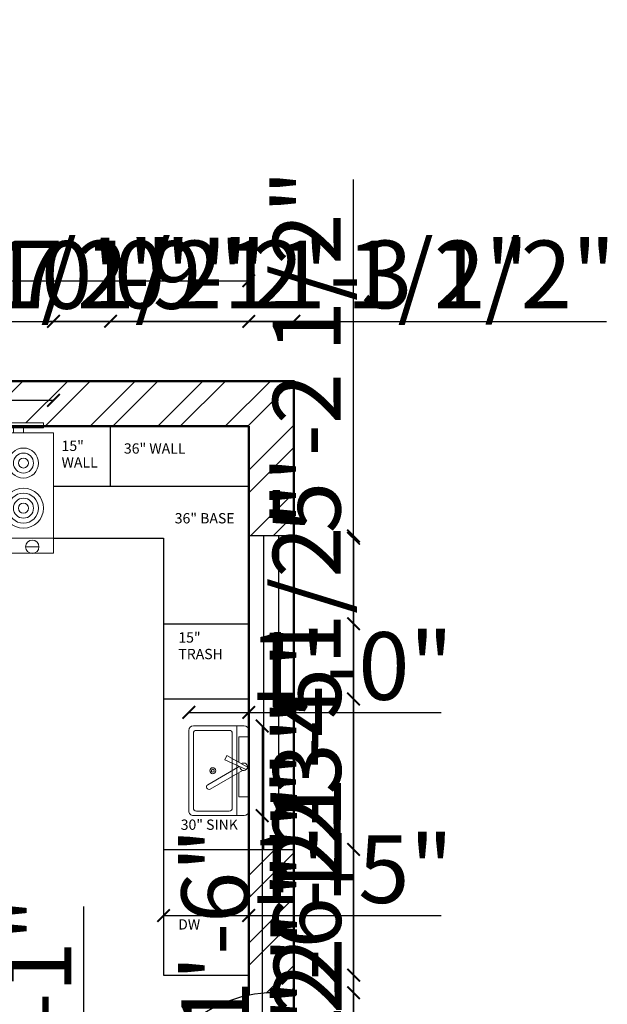
# Model space of a CAD drawing. Units: inches. Extents: x 1736 to 2023, y 1717 to 2014.
# Tile 3 of 3: x 1906 to 2023, y 1818 to 2014. Entities that reach past the tile are written whole.
import ezdxf

# ---------------------------------------------------------------- set-up
doc = ezdxf.new("R2010")
doc.units = ezdxf.units.IN
for name, color, linetype, lineweight in [('A-ANNO-DIMS', 2, 'Continuous', 18), ('A-ANNO-TEXT', 3, 'Continuous', 18), ('A-DOOR', 4, 'Continuous', 25), ('A-EQPM', 9, 'Continuous', 18), ('A-FLOR-CASE', 8, 'Continuous', 25), ('A-FLOR-FIXT', 9, 'Continuous', 18), ('A-GLAZ', 4, 'Continuous', 25), ('A-WALL', 7, 'Continuous', 50), ('A-WALL-PATT', 8, 'Continuous', 13)]:
    doc.layers.add(name, color=color, linetype=linetype, lineweight=lineweight)
doc.styles.get("Standard").update_dxf_attribs({"font": 'arial.ttf'})
doc.dimstyles.new('ISO-25', dxfattribs={"dimtxt": 13.5, "dimasz": 2.5, "dimexe": 1.25, "dimexo": 0.625, "dimtad": 1, "dimdec": 0, "dimlunit": 4, "dimtxsty": 'Standard', "dimblk": 'ARCHTICK', "dimcen": 2.5, "dimse1": 1, "dimse2": 1, "dimclrd": 2, "dimclrt": 4, "dimadec": 0, "dimazin": 0, "dimtfac": 1, "dimtdec": 0, "dimtmove": 0, "dimatfit": 3, "dimfxl": 1, "dimarcsym": 0})

# ---------------------------------------------------------------- blocks, each defined once
blk = doc.blocks.new('Range-Oven - 30 in top')
for p, q in [((0, -3), (30, -3)), ((12, -6), (18, -6)), ((13, -20), (13, -6)), ((14, -6), (14, -20)), ((15, -20), (15, -6)), ((16, -6), (16, -20)), ((17, -20), (17, -6)), ((18, -20), (12, -20)), ((6, -24), (6, -25)), ((8, -25), (8, -24)), ((22, -25), (22, -24)), ((24, -24), (24, -25))]:
    blk.add_line(p, q)
for points in [[(0, -24), (0, 0), (30, 0), (30, -24)], [(12, -21), (12, -5), (18, -5), (18, -21)], [(2, -26), (2, -25), (28, -25), (28, -26)]]:
    blk.add_lwpolyline(points, close=True)
for centre, radius in [((6, -9), 4), ((6, -9), 3), ((6, -9), 2), ((24, -9), 3), ((24, -9), 2), ((6, -9), 1), ((24, -9), 1), ((6, -18), 3), ((24, -18), 4), ((24, -18), 3), ((6, -18), 2), ((6, -18), 1), ((24, -18), 2), ((24, -18), 1)]:
    blk.add_circle(centre, radius)
blk = doc.blocks.new('*U4')
for p, q in [((0, 0), (0, -6)), ((40, 0), (40, -6))]:
    blk.add_line(p, q)
blk.add_lwpolyline([(0, 0), (0, 40), (1.75, 40), (1.75, 0)], close=True)
blk.add_arc((0, 0), 40, 0, 90)
blk = doc.blocks.new('Sink-single - 30 in top')
blk.add_line((-15, -3.999996), (15, -3.999996))
for points in [[(-13.5, 0), (13.5, 0)], [(-15, -18.499996), (-15, -1.5)], [(15, -1.5), (15, -18.499996)], [(-13.5, -17.499996), (-13.5, -6.499996)], [(-12.5, -5.499996), (12.5, -5.499996)], [(13.5, -6.499996), (13.5, -17.499996)], [(12.5, -18.499996), (-12.5, -18.499996)], [(13.5, -19.999996), (-13.5, -19.999996)]]:
    blk.add_lwpolyline(points)
for radius in [1, 0.5]:
    blk.add_circle((0, -11.999996), radius)
for centre, radius, start, end in [((-13.5, -1.5), 1.5, 90, 180), ((13.5, -1.5), 1.5, 0, 90), ((-12.5, -6.499996), 1, 90, 180), ((12.5, -6.499996), 1, 0, 90), ((-13.5, -18.499996), 1.5, 180, 270), ((-12.5, -17.499996), 1, 180, 270), ((12.5, -17.499996), 1, 270, 0), ((13.5, -18.499996), 1.5, 270, 0)]:
    blk.add_arc(centre, radius, start, end)
blk = doc.blocks.new('Faucet - single handle top')
for p, q in [((0.08, -0.26), (-2.26, -4.34)), ((-1.37, -4.79), (0.55, -0.5)), ((-0.06, -1.9), (3.57, -8.18)), ((4.43, -7.68), (0.72, -1.24)), ((-2.26, -4.34), (-1.37, -4.79))]:
    blk.add_line(p, q)
for points in [[(-0.92, -2), (-6, -2), (-6, 0), (6, 0), (6, -2), (1.16, -2)], [(-0.01, -2), (-0.12, -2)]]:
    blk.add_lwpolyline(points)
for centre, radius, start, end in [((0, -1), 0.75, 269.2246, 216.2304), ((4, -7.93), 0.5, 210, 30)]:
    blk.add_arc(centre, radius, start, end)
blk = doc.blocks.new('_ArchTick')
at = {"color": 0, "linetype": 'ByBlock', "const_width": 0.15}
blk.add_lwpolyline([(-0.5, -0.5), (0.5, 0.5)], dxfattribs=at)
blk = doc.blocks.new('*D7')
at = {"layer": 'A-ANNO-DIMS', "color": 0, "lineweight": -2, "transparency": 16777216}
blk.add_line((1831.43, 1962.29), (1951.43, 1962.29), dxfattribs=at)
at = {"layer": 'Defpoints', "color": 0, "transparency": 16777216}
for p in [(1951.43, 1962.29), (1831.43, 1933.29), (1951.43, 1933.29)]:
    blk.add_point(p, dxfattribs=at)
at = {"layer": 'A-ANNO-DIMS', "color": 0, "lineweight": -2, "transparency": 16777216, "xscale": 2.5, "yscale": 2.5, "zscale": 2.5, "rotation": 180}
blk.add_blockref('_ArchTick', (1831.43, 1962.29), dxfattribs=at)
at = {"layer": 'A-ANNO-DIMS', "color": 0, "lineweight": -2, "transparency": 16777216, "xscale": 2.5, "yscale": 2.5, "zscale": 2.5}
blk.add_blockref('_ArchTick', (1951.43, 1962.29), dxfattribs=at)
at = {"layer": 'A-ANNO-DIMS', "color": 0, "transparency": 16777216, "insert": (1891.43, 1969.8), "char_height": 13.5, "attachment_point": 5}
blk.add_mtext("10'", dxfattribs=at)
blk = doc.blocks.new('*D9')
at = {"layer": 'A-ANNO-DIMS', "color": 2, "lineweight": -2, "transparency": 16777216}
for p, q in [((1882.52, 1938.43), (1771.27, 1938.43)), ((1912.52, 1938.43), (1882.52, 1938.43))]:
    blk.add_line(p, q, dxfattribs=at)
at = {"layer": 'Defpoints', "color": 0, "transparency": 16777216}
for p in [(1882.52, 1938.43), (1882.52, 1933.93), (1912.52, 1933.93)]:
    blk.add_point(p, dxfattribs=at)
at = {"layer": 'A-ANNO-DIMS', "color": 2, "lineweight": -2, "transparency": 16777216, "xscale": 2.5, "yscale": 2.5, "zscale": 2.5, "rotation": 180}
blk.add_blockref('_ArchTick', (1882.52, 1938.43), dxfattribs=at)
at = {"layer": 'A-ANNO-DIMS', "color": 2, "lineweight": -2, "transparency": 16777216, "xscale": 2.5, "yscale": 2.5, "zscale": 2.5}
blk.add_blockref('_ArchTick', (1912.52, 1938.43), dxfattribs=at)
at = {"layer": 'A-ANNO-DIMS', "color": 4, "transparency": 16777216, "insert": (1825.64, 1946.04), "char_height": 13.5, "attachment_point": 5}
blk.add_mtext('RANGE 2\'-6"', dxfattribs=at)
blk = doc.blocks.new('*D11')
at = {"layer": 'A-ANNO-DIMS', "color": 2, "lineweight": -2, "transparency": 16777216}
for p, q in [((1954.12, 1873.5), (1954.12, 1855.61)), ((1954.12, 1855.61), (1954.12, 1766.78))]:
    blk.add_line(p, q, dxfattribs=at)
at = {"layer": 'Defpoints', "color": 0, "transparency": 16777216}
for p in [(1951.43, 1873.5), (1951.43, 1855.61), (1954.12, 1855.61)]:
    blk.add_point(p, dxfattribs=at)
at = {"layer": 'A-ANNO-DIMS', "color": 2, "lineweight": -2, "transparency": 16777216, "xscale": 2.5, "yscale": 2.5, "zscale": 2.5}
for p, rotation in [((1954.12, 1873.5), 90), ((1954.12, 1855.61), 270)]:
    blk.add_blockref('_ArchTick', p, dxfattribs=dict(at, rotation=rotation))
at = {"layer": 'A-ANNO-DIMS', "color": 4, "transparency": 16777216, "insert": (1946.51, 1809.94), "char_height": 13.5, "attachment_point": 5, "rotation": 90}
blk.add_mtext('SINK 1\'-6"', dxfattribs=at)
blk = doc.blocks.new('*D12')
at = {"layer": 'A-ANNO-DIMS', "color": 2, "lineweight": -2, "transparency": 16777216}
for p, q in [((1939.5, 1876.19), (1951.43, 1876.19)), ((1951.43, 1876.19), (1989.8, 1876.19))]:
    blk.add_line(p, q, dxfattribs=at)
at = {"layer": 'Defpoints', "color": 0, "transparency": 16777216}
for p in [(1951.43, 1876.19), (1939.5, 1873.5), (1951.43, 1873.5)]:
    blk.add_point(p, dxfattribs=at)
at = {"layer": 'A-ANNO-DIMS', "color": 2, "lineweight": -2, "transparency": 16777216, "xscale": 2.5, "yscale": 2.5, "zscale": 2.5, "rotation": 180}
blk.add_blockref('_ArchTick', (1939.5, 1876.19), dxfattribs=at)
at = {"layer": 'A-ANNO-DIMS', "color": 2, "lineweight": -2, "transparency": 16777216, "xscale": 2.5, "yscale": 2.5, "zscale": 2.5}
blk.add_blockref('_ArchTick', (1951.43, 1876.19), dxfattribs=at)
at = {"layer": 'A-ANNO-DIMS', "color": 4, "transparency": 16777216, "insert": (1971.87, 1883.7), "char_height": 13.5, "attachment_point": 5}
blk.add_mtext('1\'-0"', dxfattribs=at)
blk = doc.blocks.new('*D16')
at = {"layer": 'A-ANNO-DIMS', "color": 2, "lineweight": -2, "transparency": 16777216}
for p, q in [((1951.43, 1954.19), (1911.8, 1954.19)), ((1960.43, 1954.19), (1951.43, 1954.19))]:
    blk.add_line(p, q, dxfattribs=at)
at = {"layer": 'Defpoints', "color": 0, "transparency": 16777216}
for p in [(1951.43, 1954.19), (1960.43, 1942.29), (1951.43, 1933.29)]:
    blk.add_point(p, dxfattribs=at)
at = {"layer": 'A-ANNO-DIMS', "color": 2, "lineweight": -2, "transparency": 16777216, "xscale": 2.5, "yscale": 2.5, "zscale": 2.5, "rotation": 180}
blk.add_blockref('_ArchTick', (1951.43, 1954.19), dxfattribs=at)
at = {"layer": 'A-ANNO-DIMS', "color": 2, "lineweight": -2, "transparency": 16777216, "xscale": 2.5, "yscale": 2.5, "zscale": 2.5}
blk.add_blockref('_ArchTick', (1960.43, 1954.19), dxfattribs=at)
at = {"layer": 'A-ANNO-DIMS', "color": 4, "transparency": 16777216, "insert": (1930.36, 1961.7), "char_height": 13.5, "attachment_point": 5}
blk.add_mtext('0\'-9"', dxfattribs=at)
blk = doc.blocks.new('*D24')
at = {"layer": 'A-ANNO-DIMS', "color": 2, "lineweight": -2, "transparency": 16777216}
for p, q in [((1972.33, 1794.21), (1972.33, 1832.57)), ((1972.33, 1780.29), (1972.33, 1794.21))]:
    blk.add_line(p, q, dxfattribs=at)
at = {"layer": 'Defpoints', "color": 0, "transparency": 16777216}
for p in [(1960.43, 1794.21), (1972.33, 1794.21), (1960.43, 1780.29)]:
    blk.add_point(p, dxfattribs=at)
at = {"layer": 'A-ANNO-DIMS', "color": 2, "lineweight": -2, "transparency": 16777216, "xscale": 2.5, "yscale": 2.5, "zscale": 2.5}
for p, rotation in [((1972.33, 1794.21), 90), ((1972.33, 1780.29), 270)]:
    blk.add_blockref('_ArchTick', p, dxfattribs=dict(at, rotation=rotation))
at = {"layer": 'A-ANNO-DIMS', "color": 4, "transparency": 16777216, "insert": (1964.93, 1814.64), "char_height": 13.5, "attachment_point": 5, "rotation": 90}
blk.add_mtext('1\'-2"', dxfattribs=at)
blk = doc.blocks.new('*D25')
at = {"layer": 'A-ANNO-DIMS', "color": 2, "lineweight": -2, "transparency": 16777216}
for p, q in [((1972.33, 1820.25), (1972.33, 1860.12)), ((1972.33, 1794.21), (1972.33, 1820.25))]:
    blk.add_line(p, q, dxfattribs=at)
at = {"layer": 'Defpoints', "color": 0, "transparency": 16777216}
for p in [(1960.43, 1820.25), (1972.33, 1820.25), (1960.43, 1794.21)]:
    blk.add_point(p, dxfattribs=at)
at = {"layer": 'A-ANNO-DIMS', "color": 2, "lineweight": -2, "transparency": 16777216, "xscale": 2.5, "yscale": 2.5, "zscale": 2.5}
for p, rotation in [((1972.33, 1820.25), 90), ((1972.33, 1794.21), 270)]:
    blk.add_blockref('_ArchTick', p, dxfattribs=dict(at, rotation=rotation))
at = {"layer": 'A-ANNO-DIMS', "color": 4, "transparency": 16777216, "insert": (1964.93, 1841.44), "char_height": 13.5, "attachment_point": 5, "rotation": 90}
blk.add_mtext('2\'-2"', dxfattribs=at)
blk = doc.blocks.new('*D26')
at = {"layer": 'A-ANNO-DIMS', "color": 2, "lineweight": -2, "transparency": 16777216}
for p, q in [((1972.33, 1848.88), (1972.33, 1920.2)), ((1972.33, 1820.25), (1972.33, 1848.88))]:
    blk.add_line(p, q, dxfattribs=at)
at = {"layer": 'Defpoints', "color": 0, "transparency": 16777216}
for p in [(1960.43, 1848.88), (1972.33, 1848.88), (1960.43, 1820.25)]:
    blk.add_point(p, dxfattribs=at)
at = {"layer": 'A-ANNO-DIMS', "color": 2, "lineweight": -2, "transparency": 16777216, "xscale": 2.5, "yscale": 2.5, "zscale": 2.5}
for p, rotation in [((1972.33, 1848.88), 90), ((1972.33, 1820.25), 270)]:
    blk.add_blockref('_ArchTick', p, dxfattribs=dict(at, rotation=rotation))
at = {"layer": 'A-ANNO-DIMS', "color": 4, "transparency": 16777216, "insert": (1964.73, 1885.79), "char_height": 13.5, "attachment_point": 5, "rotation": 90}
blk.add_mtext('2\'-4 1/2"', dxfattribs=at)
blk = doc.blocks.new('*D27')
at = {"layer": 'A-ANNO-DIMS', "color": 2, "lineweight": -2, "transparency": 16777216}
for p, q in [((1972.33, 1911.39), (1972.33, 1982.49)), ((1972.33, 1848.88), (1972.33, 1911.39))]:
    blk.add_line(p, q, dxfattribs=at)
at = {"layer": 'Defpoints', "color": 0, "transparency": 16777216}
for p in [(1960.43, 1911.39), (1972.33, 1911.39), (1960.43, 1848.88)]:
    blk.add_point(p, dxfattribs=at)
at = {"layer": 'A-ANNO-DIMS', "color": 2, "lineweight": -2, "transparency": 16777216, "xscale": 2.5, "yscale": 2.5, "zscale": 2.5}
for p, rotation in [((1972.33, 1911.39), 90), ((1972.33, 1848.88), 270)]:
    blk.add_blockref('_ArchTick', p, dxfattribs=dict(at, rotation=rotation))
at = {"layer": 'A-ANNO-DIMS', "color": 4, "transparency": 16777216, "insert": (1964.73, 1948.19), "char_height": 13.5, "attachment_point": 5, "rotation": 90}
blk.add_mtext('5\'-2 1/2"', dxfattribs=at)
blk = doc.blocks.new('*D28')
at = {"layer": 'A-ANNO-DIMS', "color": 2, "lineweight": -2, "transparency": 16777216}
for p, q in [((1918.58, 1795.35), (1918.58, 1837.48)), ((1918.58, 1794.21), (1918.58, 1795.35)), ((1918.58, 1794.21), (1918.58, 1791.71))]:
    blk.add_line(p, q, dxfattribs=at)
at = {"layer": 'Defpoints', "color": 0, "transparency": 16777216}
for p in [(1918.58, 1795.35), (1930.48, 1795.35), (1930.48, 1794.21)]:
    blk.add_point(p, dxfattribs=at)
at = {"layer": 'A-ANNO-DIMS', "color": 2, "lineweight": -2, "transparency": 16777216, "xscale": 2.5, "yscale": 2.5, "zscale": 2.5}
for p, rotation in [((1918.58, 1795.35), 270), ((1918.58, 1794.21), 90)]:
    blk.add_blockref('_ArchTick', p, dxfattribs=dict(at, rotation=rotation))
at = {"layer": 'A-ANNO-DIMS', "color": 4, "transparency": 16777216, "insert": (1911.06, 1818.91), "char_height": 13.5, "attachment_point": 5, "rotation": 90}
blk.add_mtext('0\'-1"', dxfattribs=at)
blk = doc.blocks.new('*D30')
at = {"layer": 'A-ANNO-DIMS', "color": 2, "lineweight": -2, "transparency": 16777216}
for p, q in [((1763.99, 1933.29), (1763.99, 2013.6)), ((1763.99, 1910.93), (1763.99, 1933.29))]:
    blk.add_line(p, q, dxfattribs=at)
at = {"layer": 'Defpoints', "color": 0, "transparency": 16777216}
for p in [(1763.99, 1933.29), (1951.43, 1933.29), (1934.43, 1910.93)]:
    blk.add_point(p, dxfattribs=at)
at = {"layer": 'A-ANNO-DIMS', "color": 2, "lineweight": -2, "transparency": 16777216, "xscale": 2.5, "yscale": 2.5, "zscale": 2.5}
for p, rotation in [((1763.99, 1933.29), 90), ((1763.99, 1910.93), 270)]:
    blk.add_blockref('_ArchTick', p, dxfattribs=dict(at, rotation=rotation))
at = {"layer": 'A-ANNO-DIMS', "color": 4, "transparency": 16777216, "insert": (1756.39, 1974.69), "char_height": 13.5, "attachment_point": 5, "rotation": 90}
blk.add_mtext('1\'-10 1/2"', dxfattribs=at)
blk = doc.blocks.new('*D31')
at = {"layer": 'A-ANNO-DIMS', "color": 2, "lineweight": -2, "transparency": 16777216}
for p, q in [((1934.43, 1835.67), (1951.43, 1835.67)), ((1951.43, 1835.67), (1989.8, 1835.67))]:
    blk.add_line(p, q, dxfattribs=at)
at = {"layer": 'Defpoints', "color": 0, "transparency": 16777216}
for p in [(1951.43, 1835.67), (1934.43, 1823.77), (1951.43, 1823.77)]:
    blk.add_point(p, dxfattribs=at)
at = {"layer": 'A-ANNO-DIMS', "color": 2, "lineweight": -2, "transparency": 16777216, "xscale": 2.5, "yscale": 2.5, "zscale": 2.5, "rotation": 180}
blk.add_blockref('_ArchTick', (1934.43, 1835.67), dxfattribs=at)
at = {"layer": 'A-ANNO-DIMS', "color": 2, "lineweight": -2, "transparency": 16777216, "xscale": 2.5, "yscale": 2.5, "zscale": 2.5}
blk.add_blockref('_ArchTick', (1951.43, 1835.67), dxfattribs=at)
at = {"layer": 'A-ANNO-DIMS', "color": 4, "transparency": 16777216, "insert": (1971.87, 1843.18), "char_height": 13.5, "attachment_point": 5}
blk.add_mtext('1\'-5"', dxfattribs=at)
blk = doc.blocks.new('*D34')
at = {"layer": 'A-ANNO-DIMS', "color": 2, "lineweight": -2, "transparency": 16777216}
for p, q in [((1831.43, 1954.19), (1862.97, 1954.19)), ((1862.97, 1954.19), (1934.3, 1954.19))]:
    blk.add_line(p, q, dxfattribs=at)
at = {"layer": 'Defpoints', "color": 0, "transparency": 16777216}
for p in [(1862.97, 1954.19), (1831.43, 1933.29), (1862.97, 1933.29)]:
    blk.add_point(p, dxfattribs=at)
at = {"layer": 'A-ANNO-DIMS', "color": 2, "lineweight": -2, "transparency": 16777216, "xscale": 2.5, "yscale": 2.5, "zscale": 2.5, "rotation": 180}
blk.add_blockref('_ArchTick', (1831.43, 1954.19), dxfattribs=at)
at = {"layer": 'A-ANNO-DIMS', "color": 2, "lineweight": -2, "transparency": 16777216, "xscale": 2.5, "yscale": 2.5, "zscale": 2.5}
blk.add_blockref('_ArchTick', (1862.97, 1954.19), dxfattribs=at)
at = {"layer": 'A-ANNO-DIMS', "color": 4, "transparency": 16777216, "insert": (1899.89, 1961.79), "char_height": 13.5, "attachment_point": 5}
blk.add_mtext('2\'-7 1/2"', dxfattribs=at)
blk = doc.blocks.new('*D35')
at = {"layer": 'A-ANNO-DIMS', "color": 2, "lineweight": -2, "transparency": 16777216}
for p, q in [((1862.97, 1954.19), (1882.52, 1954.19)), ((1882.52, 1954.19), (1952.34, 1954.19))]:
    blk.add_line(p, q, dxfattribs=at)
at = {"layer": 'Defpoints', "color": 0, "transparency": 16777216}
for p in [(1882.52, 1954.19), (1862.97, 1921.29), (1882.52, 1921.29)]:
    blk.add_point(p, dxfattribs=at)
at = {"layer": 'A-ANNO-DIMS', "color": 2, "lineweight": -2, "transparency": 16777216, "xscale": 2.5, "yscale": 2.5, "zscale": 2.5, "rotation": 180}
blk.add_blockref('_ArchTick', (1862.97, 1954.19), dxfattribs=at)
at = {"layer": 'A-ANNO-DIMS', "color": 2, "lineweight": -2, "transparency": 16777216, "xscale": 2.5, "yscale": 2.5, "zscale": 2.5}
blk.add_blockref('_ArchTick', (1882.52, 1954.19), dxfattribs=at)
at = {"layer": 'A-ANNO-DIMS', "color": 4, "transparency": 16777216, "insert": (1918.68, 1961.79), "char_height": 13.5, "attachment_point": 5}
blk.add_mtext('1\'-7 1/2"', dxfattribs=at)
blk = doc.blocks.new('*D36')
at = {"layer": 'A-ANNO-DIMS', "color": 2, "lineweight": -2, "transparency": 16777216}
for p, q in [((1912.52, 1954.19), (1923.89, 1954.19)), ((1923.89, 1954.19), (2005.47, 1954.19))]:
    blk.add_line(p, q, dxfattribs=at)
at = {"layer": 'Defpoints', "color": 0, "transparency": 16777216}
for p in [(1923.89, 1954.19), (1912.52, 1921.29), (1923.89, 1921.29)]:
    blk.add_point(p, dxfattribs=at)
at = {"layer": 'A-ANNO-DIMS', "color": 2, "lineweight": -2, "transparency": 16777216, "xscale": 2.5, "yscale": 2.5, "zscale": 2.5, "rotation": 180}
blk.add_blockref('_ArchTick', (1912.52, 1954.19), dxfattribs=at)
at = {"layer": 'A-ANNO-DIMS', "color": 2, "lineweight": -2, "transparency": 16777216, "xscale": 2.5, "yscale": 2.5, "zscale": 2.5}
blk.add_blockref('_ArchTick', (1923.89, 1954.19), dxfattribs=at)
at = {"layer": 'A-ANNO-DIMS', "color": 4, "transparency": 16777216, "insert": (1965.93, 1961.79), "char_height": 13.5, "attachment_point": 5}
blk.add_mtext('0\'-11 1/2"', dxfattribs=at)
blk = doc.blocks.new('*D37')
at = {"layer": 'A-ANNO-DIMS', "color": 2, "lineweight": -2, "transparency": 16777216}
for p, q in [((1923.89, 1954.19), (1951.43, 1954.19)), ((1951.43, 1954.19), (2022.76, 1954.19))]:
    blk.add_line(p, q, dxfattribs=at)
at = {"layer": 'Defpoints', "color": 0, "transparency": 16777216}
for p in [(1951.43, 1954.19), (1923.89, 1921.29), (1951.43, 1921.29)]:
    blk.add_point(p, dxfattribs=at)
at = {"layer": 'A-ANNO-DIMS', "color": 2, "lineweight": -2, "transparency": 16777216, "xscale": 2.5, "yscale": 2.5, "zscale": 2.5, "rotation": 180}
blk.add_blockref('_ArchTick', (1923.89, 1954.19), dxfattribs=at)
at = {"layer": 'A-ANNO-DIMS', "color": 2, "lineweight": -2, "transparency": 16777216, "xscale": 2.5, "yscale": 2.5, "zscale": 2.5}
blk.add_blockref('_ArchTick', (1951.43, 1954.19), dxfattribs=at)
at = {"layer": 'A-ANNO-DIMS', "color": 4, "transparency": 16777216, "insert": (1988.34, 1961.8), "char_height": 13.5, "attachment_point": 5}
blk.add_mtext('2\'-3 1/2"', dxfattribs=at)
blk = doc.blocks.new('*D45')
at = {"layer": 'A-ANNO-DIMS', "color": 2, "lineweight": -2, "transparency": 16777216}
for p, q in [((1972.33, 1910.93), (1972.33, 1893.88)), ((1972.33, 1893.88), (1972.33, 1855.52))]:
    blk.add_line(p, q, dxfattribs=at)
at = {"layer": 'Defpoints', "color": 0, "transparency": 16777216}
for p in [(1934.43, 1910.93), (1934.43, 1893.88), (1972.33, 1893.88)]:
    blk.add_point(p, dxfattribs=at)
at = {"layer": 'A-ANNO-DIMS', "color": 2, "lineweight": -2, "transparency": 16777216, "xscale": 2.5, "yscale": 2.5, "zscale": 2.5}
for p, rotation in [((1972.33, 1910.93), 90), ((1972.33, 1893.88), 270)]:
    blk.add_blockref('_ArchTick', p, dxfattribs=dict(at, rotation=rotation))
at = {"layer": 'A-ANNO-DIMS', "color": 4, "transparency": 16777216, "insert": (1964.82, 1873.45), "char_height": 13.5, "attachment_point": 5, "rotation": 90}
blk.add_mtext('1\'-5"', dxfattribs=at)
blk = doc.blocks.new('*D46')
at = {"layer": 'A-ANNO-DIMS', "color": 2, "lineweight": -2, "transparency": 16777216}
for p, q in [((1972.33, 1893.88), (1972.33, 1878.88)), ((1972.33, 1878.88), (1972.33, 1840.52))]:
    blk.add_line(p, q, dxfattribs=at)
at = {"layer": 'Defpoints', "color": 0, "transparency": 16777216}
for p in [(1934.43, 1893.88), (1934.43, 1878.88), (1972.33, 1878.88)]:
    blk.add_point(p, dxfattribs=at)
at = {"layer": 'A-ANNO-DIMS', "color": 2, "lineweight": -2, "transparency": 16777216, "xscale": 2.5, "yscale": 2.5, "zscale": 2.5}
for p, rotation in [((1972.33, 1893.88), 90), ((1972.33, 1878.88), 270)]:
    blk.add_blockref('_ArchTick', p, dxfattribs=dict(at, rotation=rotation))
at = {"layer": 'A-ANNO-DIMS', "color": 4, "transparency": 16777216, "insert": (1964.81, 1858.45), "char_height": 13.5, "attachment_point": 5, "rotation": 90}
blk.add_mtext('1\'-3"', dxfattribs=at)
blk = doc.blocks.new('*D47')
at = {"layer": 'A-ANNO-DIMS', "color": 2, "lineweight": -2, "transparency": 16777216}
for p, q in [((1972.33, 1878.88), (1972.33, 1848.88)), ((1972.33, 1848.88), (1972.33, 1809.01))]:
    blk.add_line(p, q, dxfattribs=at)
at = {"layer": 'Defpoints', "color": 0, "transparency": 16777216}
for p in [(1934.43, 1878.88), (1934.43, 1848.88), (1972.33, 1848.88)]:
    blk.add_point(p, dxfattribs=at)
at = {"layer": 'A-ANNO-DIMS', "color": 2, "lineweight": -2, "transparency": 16777216, "xscale": 2.5, "yscale": 2.5, "zscale": 2.5}
for p, rotation in [((1972.33, 1878.88), 90), ((1972.33, 1848.88), 270)]:
    blk.add_blockref('_ArchTick', p, dxfattribs=dict(at, rotation=rotation))
at = {"layer": 'A-ANNO-DIMS', "color": 4, "transparency": 16777216, "insert": (1964.82, 1827.7), "char_height": 13.5, "attachment_point": 5, "rotation": 90}
blk.add_mtext('2\'-6"', dxfattribs=at)
blk = doc.blocks.new('*D48')
at = {"layer": 'A-ANNO-DIMS', "color": 2, "lineweight": -2, "transparency": 16777216}
for p, q in [((1972.33, 1848.88), (1972.33, 1823.77)), ((1972.33, 1823.77), (1972.33, 1783.9))]:
    blk.add_line(p, q, dxfattribs=at)
at = {"layer": 'Defpoints', "color": 0, "transparency": 16777216}
for p in [(1934.43, 1848.88), (1934.43, 1823.77), (1972.33, 1823.77)]:
    blk.add_point(p, dxfattribs=at)
at = {"layer": 'A-ANNO-DIMS', "color": 2, "lineweight": -2, "transparency": 16777216, "xscale": 2.5, "yscale": 2.5, "zscale": 2.5}
for p, rotation in [((1972.33, 1848.88), 90), ((1972.33, 1823.77), 270)]:
    blk.add_blockref('_ArchTick', p, dxfattribs=dict(at, rotation=rotation))
at = {"layer": 'A-ANNO-DIMS', "color": 4, "transparency": 16777216, "insert": (1964.93, 1802.58), "char_height": 13.5, "attachment_point": 5, "rotation": 90}
blk.add_mtext('2\'-1"', dxfattribs=at)

msp = doc.modelspace()

# ---------------------------------------------------------------- hatches: boundary and pattern name
at = {"layer": 'A-WALL-PATT'}
h = msp.add_hatch(dxfattribs=at)
h.set_pattern_fill('ANSI32', color=256)
h.paths.add_polyline_path([(1831.43, 1933.29), (1884.52, 1933.29), (1884.52, 1933.93), (1910.52, 1933.93), (1910.52, 1933.29), (1951.43, 1933.29), (1951.43, 1911.39), (1960.43, 1911.39), (1960.43, 1942.29), (1822.43, 1942.29), (1775.89, 1942.29), (1775.89, 1933.29), (1822.43, 1933.29), (1822.43, 1815.68), (1831.43, 1815.68)])
h.paths.add_polyline_path([(1960.43, 1848.88), (1951.43, 1848.88), (1951.43, 1819.75, -0.049233), (1956.53, 1820.25), (1960.43, 1820.25)], flags=17)
h.paths.add_polyline_path([(1960.43, 1794.21), (1956.53, 1794.21), (1951.43, 1794.21), (1951.43, 1789.29), (1903.21, 1789.29), (1903.21, 1780.29), (1960.43, 1780.29)])
h.paths.add_polyline_path([(1855.31, 1789.29), (1831.43, 1789.29), (1831.43, 1793.62), (1822.43, 1793.62), (1822.43, 1789.29), (1775.89, 1789.29), (1775.89, 1780.29), (1822.43, 1780.29), (1855.31, 1780.29)])

# ---------------------------------------------------------------- linework, layer by layer
at = {"layer": 'A-EQPM'}
msp.add_line((1906.96, 1909.23), (1909.63, 1909.23), dxfattribs=at)
msp.add_circle((1908.29, 1909.23), 1.33, dxfattribs=at)
at = {"layer": 'A-FLOR-CASE'}
for p, q in [((1923.89, 1921.29), (1923.89, 1933.29)), ((1912.52, 1921.29), (1951.43, 1921.29)), ((1912.52, 1910.93), (1934.43, 1910.93)), ((1934.43, 1910.93), (1934.43, 1823.77)), ((1934.43, 1893.88), (1951.43, 1893.88)), ((1934.43, 1878.88), (1951.43, 1878.88)), ((1934.43, 1848.88), (1951.43, 1848.88)), ((1934.43, 1823.77), (1951.43, 1823.77))]:
    msp.add_line(p, q, dxfattribs=at)
at = {"layer": 'A-GLAZ'}
for p, q in [((1960.43, 1911.39), (1951.43, 1911.39)), ((1951.43, 1911.39), (1951.43, 1848.88)), ((1954.43, 1848.88), (1954.43, 1911.39)), ((1957.43, 1848.88), (1957.43, 1911.39)), ((1960.43, 1848.88), (1960.43, 1911.39)), ((1951.43, 1848.88), (1960.43, 1848.88))]:
    msp.add_line(p, q, dxfattribs=at)
at = {"layer": 'A-WALL'}
for p, q in [((1831.43, 1933.29), (1951.43, 1933.29)), ((1951.43, 1933.29), (1951.43, 1819.75))]:
    msp.add_line(p, q, dxfattribs=at)
msp.add_lwpolyline([(1822.43, 1942.29), (1960.43, 1942.29), (1960.43, 1780.29), (1822.43, 1780.29)], dxfattribs=at)

# ---------------------------------------------------------------- block references
at = {"layer": 'A-DOOR', "xscale": 0.651221867343762, "yscale": 0.651221867343762, "zscale": 0.651221867343762, "rotation": 90}
msp.add_blockref('*U4', (1956.53, 1794.21), dxfattribs=at)
at = {"layer": 'A-EQPM', "rotation": 180}
msp.add_blockref('Range-Oven - 30 in top', (1912.52, 1907.93), dxfattribs=at)
at = {"layer": 'A-FLOR-FIXT', "xscale": 0.596450461610902, "yscale": 0.596450461610902, "zscale": 0.596450461610902, "rotation": 270}
msp.add_blockref('Sink-single - 30 in top', (1951.43, 1864.56), dxfattribs=at)
at = {"layer": 'A-FLOR-FIXT', "rotation": 270}
msp.add_blockref('Faucet - single handle top', (1951.43, 1865.34), dxfattribs=at)

# ---------------------------------------------------------------- texts
at = {"layer": 'A-ANNO-TEXT'}
for s, p in [('15"', (1914.12, 1928.34)), ('36" WALL', (1926.55, 1927.81)), ('WALL', (1914.12, 1925.04)), ('36" BASE', (1936.68, 1913.89)), ('15"', (1937.4, 1890.11)), ('TRASH', (1937.4, 1886.81)), ('30" SINK', (1937.87, 1852.77)), ('DW', (1937.36, 1832.88))]:
    msp.add_text(s, height=2.054, dxfattribs=at).set_placement(p)

# ---------------------------------------------------------------- dimensions: what is measured, and where the dimension line sits
at = {"layer": 'A-ANNO-DIMS'}
for base, p1, p2, picture, middle in [((1763.99, 1933.29), (1934.43, 1910.93), (1951.43, 1933.29), '*D30', (1756.39, 1974.69)), ((1972.33, 1911.39), (1960.43, 1848.88), (1960.43, 1911.39), '*D27', (1964.73, 1948.19)), ((1972.33, 1848.88), (1960.43, 1820.25), (1960.43, 1848.88), '*D26', (1964.73, 1885.79)), ((1972.333, 1893.8807), (1934.433, 1910.9335), (1934.433, 1893.8807), '*D45', (1964.8153, 1873.4479)), ((1972.33, 1878.88), (1934.43, 1893.88), (1934.43, 1878.88), '*D46', (1964.81, 1858.45)), ((1972.33, 1848.88), (1934.43, 1878.88), (1934.43, 1848.88), '*D47', (1964.82, 1827.7)), ((1972.33, 1820.25), (1960.43, 1794.21), (1960.43, 1820.25), '*D25', (1964.93, 1841.44)), ((1972.33, 1823.77), (1934.43, 1848.88), (1934.43, 1823.77), '*D48', (1964.93, 1802.58)), ((1918.58, 1795.35), (1930.48, 1794.21), (1930.48, 1795.35), '*D28', (1911.06, 1818.91)), ((1972.33, 1794.21), (1960.43, 1780.29), (1960.43, 1794.21), '*D24', (1964.93, 1814.64))]:
    dim = msp.add_linear_dim(base=base, p1=p1, p2=p2, angle=90, dimstyle='ISO-25', override={"dimdec": 1, "dimlfac": 1, "dimrnd": 0, "dimzin": 1, "dimdsep": 46, "dimlunit": 4, "dimfrac": 2}, dxfattribs=at)
    dim.commit()
    dim.dimension.update_dxf_attribs({"geometry": picture, "text_midpoint": middle})
for base, p1, p2, override, picture, middle in [((1862.97, 1954.19), (1831.43, 1933.29), (1862.97, 1933.29), {"dimdec": 1, "dimlfac": 1, "dimrnd": 0, "dimzin": 1, "dimdsep": 46, "dimlunit": 4, "dimfrac": 2}, '*D34', (1899.89, 1961.79)), ((1882.5156, 1954.1856), (1862.9743, 1921.2856), (1882.5156, 1921.2856), {"dimdec": 1, "dimlfac": 1, "dimrnd": 0, "dimzin": 1, "dimdsep": 46, "dimlunit": 4, "dimfrac": 2}, '*D35', (1918.6769, 1961.7909)), ((1923.89, 1954.19), (1912.52, 1921.29), (1923.89, 1921.29), {"dimdec": 1, "dimlfac": 1, "dimrnd": 0, "dimzin": 1, "dimdsep": 46, "dimlunit": 4, "dimfrac": 2}, '*D36', (1965.93, 1961.79)), ((1951.43, 1954.19), (1923.89, 1921.29), (1951.43, 1921.29), {"dimdec": 1, "dimlfac": 1, "dimrnd": 0, "dimzin": 1, "dimdsep": 46, "dimlunit": 4, "dimfrac": 2}, '*D37', (1988.34, 1961.8)), ((1951.43, 1962.29), (1831.43, 1933.29), (1951.43, 1933.29), {"dimclrd": 0, "dimclre": 0, "dimclrt": 0}, '*D7', (1891.43, 1969.8)), ((1951.43, 1954.19), (1960.43, 1942.29), (1951.43, 1933.29), {"dimdec": 1, "dimlfac": 1, "dimrnd": 0, "dimzin": 1, "dimdsep": 46, "dimlunit": 4, "dimfrac": 2}, '*D16', (1930.36, 1961.7)), ((1951.43, 1876.19), (1939.5, 1873.5), (1951.43, 1873.5), {"dimdec": 1, "dimlfac": 1, "dimrnd": 0, "dimzin": 1, "dimdsep": 46, "dimlunit": 4, "dimfrac": 2}, '*D12', (1971.87, 1883.7)), ((1951.43, 1835.67), (1934.43, 1823.77), (1951.43, 1823.77), {"dimdec": 1, "dimlfac": 1, "dimrnd": 0, "dimzin": 1, "dimdsep": 46, "dimlunit": 4, "dimfrac": 2}, '*D31', (1971.87, 1843.18))]:
    dim = msp.add_linear_dim(base=base, p1=p1, p2=p2, dimstyle='ISO-25', override=override, dxfattribs=at)
    dim.commit()
    dim.dimension.update_dxf_attribs({"geometry": picture, "text_midpoint": middle})
for base, p1, p2, angle, text, picture, middle in [((1882.52, 1938.43), (1912.52, 1933.93), (1882.52, 1933.93), 180, 'RANGE <>', '*D9', (1825.64, 1946.04)), ((1954.12, 1855.61), (1951.43, 1873.5), (1951.43, 1855.61), 270, 'SINK <>', '*D11', (1946.51, 1809.94))]:
    dim = msp.add_linear_dim(base=base, p1=p1, p2=p2, angle=angle, text=text, dimstyle='ISO-25', override={"dimdec": 1, "dimlfac": 1, "dimrnd": 0, "dimzin": 1, "dimdsep": 46, "dimlunit": 4, "dimfrac": 2}, dxfattribs=at)
    dim.commit()
    dim.dimension.update_dxf_attribs({"geometry": picture, "text_midpoint": middle})

doc.saveas('drawing.dxf')
